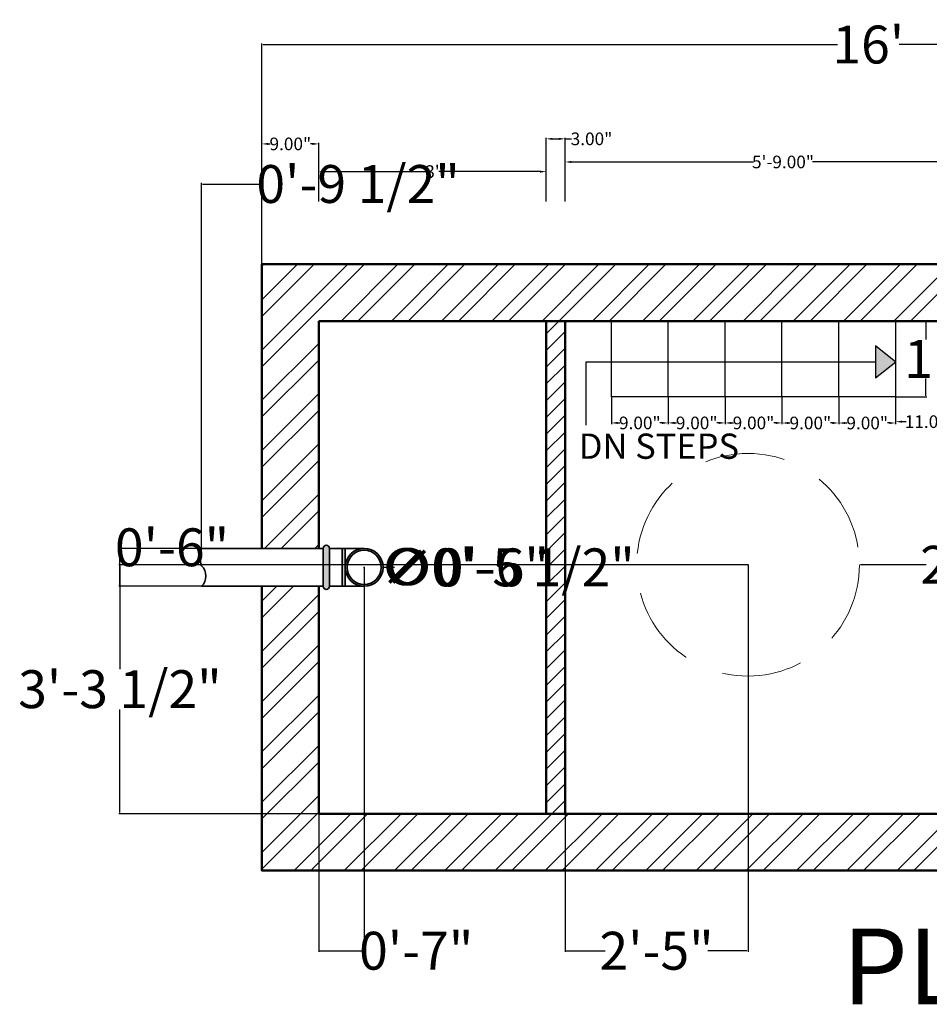
# Model space of a CAD drawing. Units: inches. Extents: x -34 to 285, y -151 to 155.
# Tile 5 of 10: x -15 to 129, y -1 to 155. Entities that reach past the tile are written whole.
import ezdxf

# ---------------------------------------------------------------- set-up
doc = ezdxf.new("R2010")
doc.units = ezdxf.units.IN
doc.header["$MEASUREMENT"] = 0
doc.linetypes.add('DASHED', pattern=[19.05, 12.7, -6.35])
for name, color, linetype, lineweight in [('A-ANNO-DIMS', 2, 'Continuous', 18), ('A-ANNO-TEXT', 7, 'Continuous', 25), ('A-DETL-HIDN', 8, 'DASHED', 18), ('A-FLOR-STRS', 3, 'Continuous', 25), ('A-WALL', 7, 'Continuous', 50), ('A-WALL-PATT', 8, 'Continuous', 18), ('P-SANR-PATT', 8, 'Continuous', 13), ('P-SANR-PIPE', 4, 'Continuous', 35)]:
    doc.layers.add(name, color=color, linetype=linetype, lineweight=lineweight)
doc.styles.get("Standard").update_dxf_attribs({"font": 'arial.ttf'})
doc.dimstyles.get("Standard").update_dxf_attribs({"dimtxt": 6, "dimasz": 0.18, "dimexe": 0.18, "dimexo": 0.0625, "dimgap": 0.09, "dimtad": 0, "dimtih": 1, "dimtoh": 1, "dimzin": 0, "dimdsep": 46, "dimlunit": 3, "dimtxsty": 'Standard', "dimcen": 0.09, "dimadec": 0, "dimazin": 0, "dimtfac": 1, "dimtofl": 0, "dimtmove": 0, "dimatfit": 3, "dimfxl": 1, "dimtolj": 1, "dimtzin": 0, "dimarcsym": 0})

# ---------------------------------------------------------------- blocks, each defined once
blk = doc.blocks.new('*D7')
at = {"layer": 'A-ANNO-DIMS', "color": 0, "lineweight": -2, "transparency": 16777216}
for p, q in [((123.25, 106.98), (128.12, 106.98)), ((127.94, 106.8), (127.94, 104.08)), ((127.94, 95.16), (127.94, 97.88)), ((123.25, 94.98), (128.12, 94.98))]:
    blk.add_line(p, q, dxfattribs=at)
at = {"layer": 'A-ANNO-DIMS', "color": 0, "transparency": 16777216}
for points in [[(127.91, 106.8), (127.97, 106.8), (127.94, 106.98)], [(127.91, 95.16), (127.97, 95.16), (127.94, 94.98)]]:
    blk.add_solid(points, dxfattribs=at)
at = {"layer": 'Defpoints', "color": 0, "transparency": 16777216}
for p in [(123.18, 106.98), (123.18, 94.98), (127.94, 94.98)]:
    blk.add_point(p, dxfattribs=at)
at = {"layer": 'A-ANNO-DIMS', "color": 0, "transparency": 16777216, "insert": (127.94, 100.98), "char_height": 6, "attachment_point": 5}
blk.add_mtext("\\A1;1'", dxfattribs=at)
blk = doc.blocks.new('*D8')
at = {"layer": 'A-ANNO-DIMS', "color": 0, "lineweight": -2, "transparency": 16777216}
for p, q in [((114.18, 94.92), (114.18, 90.66)), ((123.18, 94.92), (123.18, 90.66)), ((115.18, 90.84), (115.5, 90.84)), ((122.18, 90.84), (121.87, 90.84))]:
    blk.add_line(p, q, dxfattribs=at)
at = {"layer": 'A-ANNO-DIMS', "color": 0, "transparency": 16777216}
for points in [[(115.18, 91), (115.18, 90.67), (114.18, 90.84)], [(122.18, 91), (122.18, 90.67), (123.18, 90.84)]]:
    blk.add_solid(points, dxfattribs=at)
at = {"layer": 'Defpoints', "color": 0, "transparency": 16777216}
for p in [(114.18, 94.98), (123.18, 94.98), (114.18, 90.84)]:
    blk.add_point(p, dxfattribs=at)
at = {"layer": 'A-ANNO-DIMS', "color": 0, "transparency": 16777216, "insert": (118.68, 90.84), "char_height": 2, "attachment_point": 5}
blk.add_mtext('\\A1;9.00"', dxfattribs=at)
blk = doc.blocks.new('*D9')
at = {"layer": 'A-ANNO-DIMS', "color": 0, "lineweight": -2, "transparency": 16777216}
for p, q in [((105.18, 94.92), (105.18, 90.66)), ((114.18, 94.92), (114.18, 90.66)), ((106.18, 90.84), (106.5, 90.84)), ((113.18, 90.84), (112.87, 90.84))]:
    blk.add_line(p, q, dxfattribs=at)
at = {"layer": 'A-ANNO-DIMS', "color": 0, "transparency": 16777216}
for points in [[(106.18, 91), (106.18, 90.67), (105.18, 90.84)], [(113.18, 91), (113.18, 90.67), (114.18, 90.84)]]:
    blk.add_solid(points, dxfattribs=at)
at = {"layer": 'Defpoints', "color": 0, "transparency": 16777216}
for p in [(105.18, 94.98), (114.18, 94.98), (114.18, 90.84)]:
    blk.add_point(p, dxfattribs=at)
at = {"layer": 'A-ANNO-DIMS', "color": 0, "transparency": 16777216, "insert": (109.68, 90.84), "char_height": 2, "attachment_point": 5}
blk.add_mtext('\\A1;9.00"', dxfattribs=at)
blk = doc.blocks.new('*D10')
at = {"layer": 'A-ANNO-DIMS', "color": 0, "lineweight": -2, "transparency": 16777216}
for p, q in [((96.18, 94.92), (96.18, 90.67)), ((105.18, 94.92), (105.18, 90.67)), ((97.18, 90.85), (97.5, 90.85)), ((104.18, 90.85), (103.87, 90.85))]:
    blk.add_line(p, q, dxfattribs=at)
at = {"layer": 'A-ANNO-DIMS', "color": 0, "transparency": 16777216}
for points in [[(97.18, 91.02), (97.18, 90.68), (96.18, 90.85)], [(104.18, 91.02), (104.18, 90.68), (105.18, 90.85)]]:
    blk.add_solid(points, dxfattribs=at)
at = {"layer": 'Defpoints', "color": 0, "transparency": 16777216}
for p in [(96.18, 94.98), (105.18, 94.98), (96.18, 90.85)]:
    blk.add_point(p, dxfattribs=at)
at = {"layer": 'A-ANNO-DIMS', "color": 0, "transparency": 16777216, "insert": (100.68, 90.85), "char_height": 2, "attachment_point": 5}
blk.add_mtext('\\A1;9.00"', dxfattribs=at)
blk = doc.blocks.new('*D11')
at = {"layer": 'A-ANNO-DIMS', "color": 0, "lineweight": -2, "transparency": 16777216}
for p, q in [((87.18, 94.92), (87.18, 90.67)), ((96.18, 94.92), (96.18, 90.67)), ((88.18, 90.85), (88.5, 90.85)), ((95.18, 90.85), (94.87, 90.85))]:
    blk.add_line(p, q, dxfattribs=at)
at = {"layer": 'A-ANNO-DIMS', "color": 0, "transparency": 16777216}
for points in [[(88.18, 91.02), (88.18, 90.68), (87.18, 90.85)], [(95.18, 91.02), (95.18, 90.68), (96.18, 90.85)]]:
    blk.add_solid(points, dxfattribs=at)
at = {"layer": 'Defpoints', "color": 0, "transparency": 16777216}
for p in [(87.18, 94.98), (96.18, 94.98), (96.18, 90.85)]:
    blk.add_point(p, dxfattribs=at)
at = {"layer": 'A-ANNO-DIMS', "color": 0, "transparency": 16777216, "insert": (91.68, 90.85), "char_height": 2, "attachment_point": 5}
blk.add_mtext('\\A1;9.00"', dxfattribs=at)
blk = doc.blocks.new('*D12')
at = {"layer": 'A-ANNO-DIMS', "color": 0, "lineweight": -2, "transparency": 16777216}
for p, q in [((78.18, 94.92), (78.18, 90.67)), ((87.18, 94.92), (87.18, 90.67)), ((79.18, 90.85), (79.5, 90.85)), ((86.18, 90.85), (85.87, 90.85))]:
    blk.add_line(p, q, dxfattribs=at)
at = {"layer": 'A-ANNO-DIMS', "color": 0, "transparency": 16777216}
for points in [[(79.18, 91.02), (79.18, 90.68), (78.18, 90.85)], [(86.18, 91.02), (86.18, 90.68), (87.18, 90.85)]]:
    blk.add_solid(points, dxfattribs=at)
at = {"layer": 'Defpoints', "color": 0, "transparency": 16777216}
for p in [(78.18, 94.98), (87.18, 94.98), (78.18, 90.85)]:
    blk.add_point(p, dxfattribs=at)
at = {"layer": 'A-ANNO-DIMS', "color": 0, "transparency": 16777216, "insert": (82.68, 90.85), "char_height": 2, "attachment_point": 5}
blk.add_mtext('\\A1;9.00"', dxfattribs=at)
blk = doc.blocks.new('*D13')
at = {"layer": 'A-ANNO-DIMS', "color": 0, "lineweight": -2, "transparency": 16777216}
for p, q in [((123.18, 94.92), (123.18, 90.87)), ((134.18, 94.92), (134.18, 90.87)), ((124.18, 91.05), (124.82, 91.05)), ((133.18, 91.05), (132.55, 91.05))]:
    blk.add_line(p, q, dxfattribs=at)
at = {"layer": 'A-ANNO-DIMS', "color": 0, "transparency": 16777216}
for points in [[(124.18, 91.22), (124.18, 90.88), (123.18, 91.05)], [(133.18, 91.22), (133.18, 90.88), (134.18, 91.05)]]:
    blk.add_solid(points, dxfattribs=at)
at = {"layer": 'Defpoints', "color": 0, "transparency": 16777216}
for p in [(123.18, 94.98), (134.18, 94.98), (134.18, 91.05)]:
    blk.add_point(p, dxfattribs=at)
at = {"layer": 'A-ANNO-DIMS', "color": 0, "transparency": 16777216, "insert": (128.68, 91.05), "char_height": 2, "attachment_point": 5}
blk.add_mtext('\\A1;11.00"', dxfattribs=at)
blk = doc.blocks.new('*D14')
at = {"layer": 'A-ANNO-DIMS', "color": 0, "lineweight": -2, "transparency": 16777216}
for p, q in [((22.85, 125.9), (22.85, 135.21)), ((23.85, 135.03), (24.16, 135.03)), ((30.85, 135.03), (30.53, 135.03)), ((31.85, 125.9), (31.85, 135.21))]:
    blk.add_line(p, q, dxfattribs=at)
at = {"layer": 'A-ANNO-DIMS', "color": 0, "transparency": 16777216}
for points in [[(23.85, 135.2), (23.85, 134.86), (22.85, 135.03)], [(30.85, 135.2), (30.85, 134.86), (31.85, 135.03)]]:
    blk.add_solid(points, dxfattribs=at)
at = {"layer": 'Defpoints', "color": 0, "transparency": 16777216}
for p in [(31.85, 135.03), (22.85, 125.83), (31.85, 125.83)]:
    blk.add_point(p, dxfattribs=at)
at = {"layer": 'A-ANNO-DIMS', "color": 0, "transparency": 16777216, "insert": (27.35, 135.03), "char_height": 2, "attachment_point": 5}
blk.add_mtext('\\A1;9.00"', dxfattribs=at)
blk = doc.blocks.new('*D15')
at = {"layer": 'A-ANNO-DIMS', "color": 0, "lineweight": -2, "transparency": 16777216}
for p, q in [((31.85, 125.9), (31.85, 130.82)), ((32.85, 130.64), (48.84, 130.64)), ((66.85, 130.64), (50.86, 130.64)), ((67.85, 125.9), (67.85, 130.82))]:
    blk.add_line(p, q, dxfattribs=at)
at = {"layer": 'A-ANNO-DIMS', "color": 0, "transparency": 16777216}
for points in [[(32.85, 130.81), (32.85, 130.47), (31.85, 130.64)], [(66.85, 130.81), (66.85, 130.47), (67.85, 130.64)]]:
    blk.add_solid(points, dxfattribs=at)
at = {"layer": 'Defpoints', "color": 0, "transparency": 16777216}
for p in [(67.85, 130.64), (31.85, 125.83), (67.85, 125.83)]:
    blk.add_point(p, dxfattribs=at)
at = {"layer": 'A-ANNO-DIMS', "color": 0, "transparency": 16777216, "insert": (49.85, 130.64), "char_height": 2, "attachment_point": 5}
blk.add_mtext("\\A1;3'", dxfattribs=at)
blk = doc.blocks.new('*D16')
at = {"layer": 'A-ANNO-DIMS', "color": 0, "lineweight": -2, "transparency": 16777216}
for p, q in [((67.85, 125.9), (67.85, 136.01)), ((68.85, 135.83), (69.85, 135.83)), ((70.85, 125.9), (70.85, 136.01)), ((70.85, 135.83), (71.85, 135.83))]:
    blk.add_line(p, q, dxfattribs=at)
at = {"layer": 'A-ANNO-DIMS', "color": 0, "transparency": 16777216}
for points in [[(68.85, 135.99), (68.85, 135.66), (67.85, 135.83)], [(69.85, 135.99), (69.85, 135.66), (70.85, 135.83)]]:
    blk.add_solid(points, dxfattribs=at)
at = {"layer": 'Defpoints', "color": 0, "transparency": 16777216}
for p in [(70.85, 135.83), (67.85, 125.83), (70.85, 125.83)]:
    blk.add_point(p, dxfattribs=at)
at = {"layer": 'A-ANNO-DIMS', "color": 0, "transparency": 16777216, "insert": (75.03, 135.83), "char_height": 2, "attachment_point": 5}
blk.add_mtext('\\A1;3.00"', dxfattribs=at)
blk = doc.blocks.new('*D17')
at = {"layer": 'A-ANNO-DIMS', "color": 0, "lineweight": -2, "transparency": 16777216}
for p, q in [((70.85, 125.9), (70.85, 132.35)), ((71.85, 132.17), (100.66, 132.17)), ((138.85, 132.17), (110.04, 132.17)), ((139.85, 125.9), (139.85, 132.35))]:
    blk.add_line(p, q, dxfattribs=at)
at = {"layer": 'A-ANNO-DIMS', "color": 0, "transparency": 16777216}
for points in [[(71.85, 132.33), (71.85, 132), (70.85, 132.17)], [(138.85, 132.33), (138.85, 132), (139.85, 132.17)]]:
    blk.add_solid(points, dxfattribs=at)
at = {"layer": 'Defpoints', "color": 0, "transparency": 16777216}
for p in [(139.85, 132.17), (70.85, 125.83), (139.85, 125.83)]:
    blk.add_point(p, dxfattribs=at)
at = {"layer": 'A-ANNO-DIMS', "color": 0, "transparency": 16777216, "insert": (105.35, 132.17), "char_height": 2, "attachment_point": 5}
blk.add_mtext('\\A1;5\'-9.00"', dxfattribs=at)
blk = doc.blocks.new('*D21')
at = {"layer": 'A-ANNO-DIMS', "color": 0, "lineweight": -2, "transparency": 16777216}
for p, q in [((22.85, 130.62), (22.85, 150.94)), ((23.03, 150.76), (113.95, 150.76)), ((214.67, 150.76), (123.74, 150.76)), ((214.85, 127.74), (214.85, 150.94))]:
    blk.add_line(p, q, dxfattribs=at)
at = {"layer": 'A-ANNO-DIMS', "color": 0, "transparency": 16777216}
for points in [[(23.03, 150.79), (23.03, 150.73), (22.85, 150.76)], [(214.67, 150.79), (214.67, 150.73), (214.85, 150.76)]]:
    blk.add_solid(points, dxfattribs=at)
at = {"layer": 'Defpoints', "color": 0, "transparency": 16777216}
for p in [(22.85, 150.76), (22.85, 130.55), (214.85, 127.68)]:
    blk.add_point(p, dxfattribs=at)
at = {"layer": 'A-ANNO-DIMS', "color": 0, "transparency": 16777216, "insert": (118.85, 150.76), "char_height": 6, "attachment_point": 5}
blk.add_mtext("\\A1;16'", dxfattribs=at)
blk = doc.blocks.new('*D40')
at = {"layer": 'A-ANNO-DIMS', "color": 0, "lineweight": -2, "transparency": 16777216}
for p, q in [((99.81, 68.33), (99.81, 7.1)), ((70.85, 28.92), (70.85, 7.1)), ((71.03, 7.28), (77.21, 7.28)), ((99.63, 7.28), (93.45, 7.28))]:
    blk.add_line(p, q, dxfattribs=at)
at = {"layer": 'A-ANNO-DIMS', "color": 0, "transparency": 16777216}
for points in [[(71.03, 7.31), (71.03, 7.25), (70.85, 7.28)], [(99.63, 7.31), (99.63, 7.25), (99.81, 7.28)]]:
    blk.add_solid(points, dxfattribs=at)
at = {"layer": 'Defpoints', "color": 0, "transparency": 16777216}
for p in [(99.81, 68.39), (70.85, 28.98), (99.81, 7.28)]:
    blk.add_point(p, dxfattribs=at)
at = {"layer": 'A-ANNO-DIMS', "color": 0, "transparency": 16777216, "insert": (85.33, 7.28), "char_height": 6, "attachment_point": 5}
blk.add_mtext('\\A1;2\'-5"', dxfattribs=at)
blk = doc.blocks.new('*D42')
at = {"layer": 'A-ANNO-DIMS', "color": 0, "lineweight": -2, "transparency": 16777216}
for p, q in [((99.75, 68.39), (0.19, 68.39)), ((0.37, 68.21), (0.37, 51.88)), ((0.37, 29.16), (0.37, 45.49)), ((70.78, 28.98), (0.19, 28.98))]:
    blk.add_line(p, q, dxfattribs=at)
at = {"layer": 'A-ANNO-DIMS', "color": 0, "transparency": 16777216}
for points in [[(0.34, 68.21), (0.4, 68.21), (0.37, 68.39)], [(0.34, 29.16), (0.4, 29.16), (0.37, 28.98)]]:
    blk.add_solid(points, dxfattribs=at)
at = {"layer": 'Defpoints', "color": 0, "transparency": 16777216}
for p in [(0.37, 68.39), (99.81, 68.39), (70.85, 28.98)]:
    blk.add_point(p, dxfattribs=at)
at = {"layer": 'A-ANNO-DIMS', "color": 0, "transparency": 16777216, "insert": (0.37, 48.69), "char_height": 6, "attachment_point": 5}
blk.add_mtext('\\A1;3\'-3 1/2"', dxfattribs=at)
blk = doc.blocks.new('*D43')
at = {"layer": 'A-ANNO-DIMS', "color": 0, "lineweight": -2, "transparency": 16777216}
for p, q in [((39.04, 67.92), (39.04, 7.1)), ((31.85, 28.92), (31.85, 7.1)), ((32.03, 7.28), (38.86, 7.28)), ((39.04, 7.28), (39.22, 7.28))]:
    blk.add_line(p, q, dxfattribs=at)
at = {"layer": 'A-ANNO-DIMS', "color": 0, "transparency": 16777216}
for points in [[(32.03, 7.31), (32.03, 7.25), (31.85, 7.28)], [(38.86, 7.31), (38.86, 7.25), (39.04, 7.28)]]:
    blk.add_solid(points, dxfattribs=at)
at = {"layer": 'Defpoints', "color": 0, "transparency": 16777216}
for p in [(39.04, 67.98), (31.85, 28.98), (39.04, 7.28)]:
    blk.add_point(p, dxfattribs=at)
at = {"layer": 'A-ANNO-DIMS', "color": 0, "transparency": 16777216, "insert": (47.28, 7.28), "char_height": 6, "attachment_point": 5}
blk.add_mtext('\\A1;0\'-7"', dxfattribs=at)
blk = doc.blocks.new('*D46')
at = {"layer": 'A-ANNO-DIMS', "color": 0, "lineweight": -2, "transparency": 16777216}
for p, q in [((13.22, 70.98), (0.19, 70.98)), ((0.37, 70.98), (0.37, 71.16)), ((0.37, 71.16), (0.55, 71.16)), ((0.37, 65.16), (0.37, 70.8)), ((13.22, 64.98), (0.19, 64.98))]:
    blk.add_line(p, q, dxfattribs=at)
at = {"layer": 'A-ANNO-DIMS', "color": 0, "transparency": 16777216}
for points in [[(0.34, 70.8), (0.4, 70.8), (0.37, 70.98)], [(0.34, 65.16), (0.4, 65.16), (0.37, 64.98)]]:
    blk.add_solid(points, dxfattribs=at)
at = {"layer": 'Defpoints', "color": 0, "transparency": 16777216}
for p in [(0.37, 70.98), (13.29, 70.98), (13.29, 64.98)]:
    blk.add_point(p, dxfattribs=at)
at = {"layer": 'A-ANNO-DIMS', "color": 0, "transparency": 16777216, "insert": (8.62, 71.16), "char_height": 6, "attachment_point": 5}
blk.add_mtext('\\A1;0\'-6"', dxfattribs=at)
blk = doc.blocks.new('*D47')
at = {"layer": 'A-ANNO-DIMS', "color": 0, "lineweight": -2, "transparency": 16777216}
for p, q in [((13.29, 71.04), (13.29, 128.86)), ((13.47, 128.68), (22.67, 128.68)), ((22.85, 71.04), (22.85, 128.86)), ((22.85, 128.68), (23.03, 128.68))]:
    blk.add_line(p, q, dxfattribs=at)
at = {"layer": 'A-ANNO-DIMS', "color": 0, "transparency": 16777216}
for points in [[(13.47, 128.71), (13.47, 128.65), (13.29, 128.68)], [(22.67, 128.71), (22.67, 128.65), (22.85, 128.68)]]:
    blk.add_solid(points, dxfattribs=at)
at = {"layer": 'Defpoints', "color": 0, "transparency": 16777216}
for p in [(22.85, 128.68), (13.29, 70.98), (22.85, 70.98)]:
    blk.add_point(p, dxfattribs=at)
at = {"layer": 'A-ANNO-DIMS', "color": 0, "transparency": 16777216, "insert": (38.08, 128.68), "char_height": 6, "attachment_point": 5}
blk.add_mtext('\\A1;0\'-9 1/2"', dxfattribs=at)
blk = doc.blocks.new('*D88')
at = {"layer": 'A-ANNO-DIMS', "color": 0, "lineweight": -2, "transparency": 16777216}
for p, q in [((99.72, 68.39), (99.9, 68.39)), ((99.81, 68.3), (99.81, 68.48)), ((128.01, 68.39), (117.62, 68.39))]:
    blk.add_line(p, q, dxfattribs=at)
at = {"layer": 'A-ANNO-DIMS', "color": 0, "transparency": 16777216}
blk.add_solid([(117.62, 68.42), (117.62, 68.36), (117.44, 68.39)], dxfattribs=at)
at = {"layer": 'Defpoints', "color": 0, "transparency": 16777216}
for p in [(82.19, 68.39), (117.44, 68.39)]:
    blk.add_point(p, dxfattribs=at)
at = {"layer": 'A-ANNO-DIMS', "color": 0, "transparency": 16777216, "insert": (148.01, 68.39), "char_height": 6, "attachment_point": 5}
blk.add_mtext('\\A1;2X ∅2\'-11"', dxfattribs=at)
blk = doc.blocks.new('*D89')
at = {"layer": 'A-ANNO-DIMS', "color": 0, "lineweight": -2, "transparency": 16777216}
for p, q in [((38.95, 67.98), (39.13, 67.98)), ((39.04, 67.89), (39.04, 68.07)), ((43.84, 67.98), (42.22, 67.98))]:
    blk.add_line(p, q, dxfattribs=at)
at = {"layer": 'A-ANNO-DIMS', "color": 0, "transparency": 16777216}
blk.add_solid([(42.22, 68.01), (42.22, 67.95), (42.04, 67.98)], dxfattribs=at)
at = {"layer": 'Defpoints', "color": 0, "transparency": 16777216}
for p in [(36.04, 67.98), (42.04, 67.98)]:
    blk.add_point(p, dxfattribs=at)
at = {"layer": 'A-ANNO-DIMS', "color": 0, "transparency": 16777216, "insert": (55.16, 67.98), "char_height": 6, "attachment_point": 5}
blk.add_mtext('\\A1;∅0\'-6"', dxfattribs=at)
blk = doc.blocks.new('*D90')
at = {"layer": 'A-ANNO-DIMS', "color": 0, "lineweight": -2, "transparency": 16777216}
for p, q in [((38.95, 67.98), (39.13, 67.98)), ((39.04, 67.89), (39.04, 68.07)), ((43.36, 67.98), (41.92, 67.98))]:
    blk.add_line(p, q, dxfattribs=at)
at = {"layer": 'A-ANNO-DIMS', "color": 0, "transparency": 16777216}
blk.add_solid([(41.92, 68.01), (41.92, 67.95), (41.74, 67.98)], dxfattribs=at)
at = {"layer": 'Defpoints', "color": 0, "transparency": 16777216}
for p in [(36.34, 67.98), (41.74, 67.98)]:
    blk.add_point(p, dxfattribs=at)
at = {"layer": 'A-ANNO-DIMS', "color": 0, "transparency": 16777216, "insert": (61.68, 67.98), "char_height": 6, "attachment_point": 5}
blk.add_mtext('\\A1;∅0\'-5 1/2"', dxfattribs=at)

msp = doc.modelspace()

# ---------------------------------------------------------------- hatches: boundary and pattern name
at = {"layer": 'A-FLOR-STRS'}
h = msp.add_hatch(color=256, dxfattribs=at)
h.dxf.hatch_style = 1
h.paths.add_polyline_path([(123.184, 100.48), (120.012, 103.037), (120.012, 97.923)])
at = {"layer": 'A-WALL-PATT'}
h = msp.add_hatch(dxfattribs=at)
h.set_pattern_fill('ANSI32', color=256, scale=15)
h.paths.add_polyline_path([(214.846, 64.981), (205.846, 64.981), (205.846, 64.112), (205.846, 28.981), (31.846, 28.981), (31.846, 64.981), (22.846, 64.981), (22.846, 19.981), (214.846, 19.981)])
h.paths.add_polyline_path([(67.846, 106.981), (67.846, 115.981), (22.846, 115.981), (22.846, 70.981), (31.846, 70.981), (31.846, 106.981)])
h = msp.add_hatch(dxfattribs=at)
h.set_pattern_fill('ANSI32', color=256, scale=15)
h.paths.add_polyline_path([(214.846, 115.981), (22.846, 115.981), (22.846, 70.981), (31.846, 70.981), (31.846, 106.981), (205.846, 106.981), (205.846, 70.981), (214.846, 70.981)])
h = msp.add_hatch(dxfattribs=at)
h.set_pattern_fill('ANSI31', color=256, scale=15)
h.paths.add_polyline_path([(70.846, 106.981), (67.846, 106.981), (67.846, 28.981), (70.846, 28.981)])
at = {"layer": 'P-SANR-PATT'}
h = msp.add_hatch(color=256, dxfattribs=at)
h.dxf.hatch_style = 1
h.paths.add_polyline_path([(33.536, 70.981, 1), (32.536, 70.981), (32.536, 64.981, 1), (33.536, 64.981)])
h = msp.add_hatch(color=256, dxfattribs=at)
h.dxf.hatch_style = 1
h.paths.add_polyline_path([(36.036, 70.981), (35.536, 70.981), (35.536, 64.981), (36.036, 64.981)])
h = msp.add_hatch(color=256, dxfattribs=at)
h.dxf.hatch_style = 1
h.paths.add_polyline_path([(36.036, 67.981, 1), (42.036, 67.981, 1)])
h.paths.add_polyline_path([(41.736, 67.981, -1), (36.336, 67.981, -1)], flags=16)

# ---------------------------------------------------------------- linework, layer by layer
at = {"layer": 'A-DETL-HIDN'}
msp.add_circle((99.814, 68.391), 17.624, dxfattribs=at)
at = {"layer": 'A-FLOR-STRS'}
for p, q in [((78.184, 94.981), (78.184, 106.981)), ((87.184, 94.981), (87.184, 106.981)), ((96.184, 94.981), (96.184, 106.981)), ((105.184, 94.981), (105.184, 106.981)), ((114.184, 94.981), (114.184, 106.981)), ((123.184, 94.981), (123.184, 106.981)), ((123.184, 100.48), (120.012, 103.037)), ((120.012, 103.037), (120.012, 97.923)), ((120.012, 100.48), (74.124, 100.48)), ((74.124, 100.48), (74.124, 90.5)), ((123.184, 100.48), (120.012, 97.923))]:
    msp.add_line(p, q, dxfattribs=at)
msp.add_lwpolyline([(123.184, 94.981), (78.184, 94.981)], dxfattribs=at)
at = {"layer": 'A-WALL'}
for points in [[(22.846, 64.981), (22.846, 19.981), (214.846, 19.981), (214.846, 115.981), (22.846, 115.981), (22.846, 70.981)], [(31.846, 106.981), (31.846, 70.981)], [(205.846, 106.981), (31.846, 106.981)], [(67.846, 106.981), (67.846, 28.981)], [(70.846, 106.981), (70.846, 28.981)], [(31.846, 64.981), (31.846, 28.981)], [(31.846, 28.981), (214.846, 28.981)]]:
    msp.add_lwpolyline(points, dxfattribs=at)
at = {"layer": 'P-SANR-PIPE'}
for p, q in [((22.846, 70.981), (32.536, 70.981)), ((32.536, 70.981), (32.536, 64.981)), ((33.536, 70.981), (33.536, 64.981)), ((33.536, 70.981), (39.036, 70.981)), ((35.536, 70.981), (35.536, 64.981)), ((36.036, 70.981), (36.036, 64.981)), ((22.846, 64.981), (32.536, 64.981)), ((33.536, 64.981), (39.036, 64.981))]:
    msp.add_line(p, q, dxfattribs=at)
msp.add_lwpolyline([(13.286, 64.981, 0.4260379), (13.3, 68.24, -0.1623), (13.286, 70.981)], format="xyb", dxfattribs=at)
for points in [[(22.846, 70.981), (13.286, 70.981)], [(13.286, 64.981), (22.846, 64.981)]]:
    msp.add_lwpolyline(points, dxfattribs=at)
for radius in [3, 2.7]:
    msp.add_circle((39.036, 67.981), radius, dxfattribs=at)
for centre, start, end in [((33.036, 70.981), 0, 180), ((33.036, 64.981), 180, 0)]:
    msp.add_arc(centre, 0.5, start, end, dxfattribs=at)

# ---------------------------------------------------------------- texts
at = {"layer": 'A-ANNO-TEXT', "attachment_point": 1}
for s, insert, char_height in [('DN STEPS', (73.024, 89.167), 4), ('PLAN ', (114.748, 10.798), 12)]:
    msp.add_mtext_dynamic_manual_height_columns(s, width=53.60251, gutter_width=1, heights=[0], dxfattribs=dict(at, insert=insert, char_height=char_height))

# ---------------------------------------------------------------- dimensions: what is measured, and where the dimension line sits
at = {"layer": 'A-ANNO-DIMS'}
for base, p1, p2, override, picture, middle in [((22.846, 150.759), (214.846, 127.681), (22.846, 130.553), {"dimclrd": 0, "dimclre": 0, "dimclrt": 0}, '*D21', (118.846, 150.759)), ((22.846, 128.681), (13.286, 70.981), (22.846, 70.981), {"dimdec": 1, "dimlfac": 1, "dimrnd": 0, "dimzin": 1, "dimdsep": 46, "dimlunit": 4, "dimfrac": 2}, '*D47', (38.081, 128.681)), ((31.846, 135.03), (22.846, 125.833), (31.846, 125.833), {"dimtxt": 2, "dimasz": 1, "dimclrd": 0, "dimclre": 0, "dimclrt": 0}, '*D14', (27.346, 135.03)), ((70.846, 135.828), (67.846, 125.833), (70.846, 125.833), {"dimtxt": 2, "dimasz": 1, "dimclrd": 0, "dimclre": 0, "dimclrt": 0}, '*D16', (75.026, 135.828)), ((139.846, 132.167), (70.846, 125.833), (139.846, 125.833), {"dimtxt": 2, "dimasz": 1, "dimclrd": 0, "dimclre": 0, "dimclrt": 0}, '*D17', (105.346, 132.167)), ((67.846, 130.641), (31.846, 125.833), (67.846, 125.833), {"dimtxt": 2, "dimasz": 1, "dimclrd": 0, "dimclre": 0, "dimclrt": 0}, '*D15', (49.846, 130.641)), ((78.184, 90.851), (87.184, 94.981), (78.184, 94.981), {"dimtxt": 2, "dimasz": 1, "dimclrd": 0, "dimclre": 0, "dimclrt": 0}, '*D12', (82.684, 90.851)), ((96.184, 90.851), (87.184, 94.981), (96.184, 94.981), {"dimtxt": 2, "dimasz": 1, "dimclrd": 0, "dimclre": 0, "dimclrt": 0}, '*D11', (91.684, 90.851)), ((96.184, 90.851), (105.184, 94.981), (96.184, 94.981), {"dimtxt": 2, "dimasz": 1, "dimclrd": 0, "dimclre": 0, "dimclrt": 0}, '*D10', (100.684, 90.851)), ((114.184, 90.836), (105.184, 94.981), (114.184, 94.981), {"dimtxt": 2, "dimasz": 1, "dimclrd": 0, "dimclre": 0, "dimclrt": 0}, '*D9', (109.684, 90.836)), ((114.184, 90.836), (123.184, 94.981), (114.184, 94.981), {"dimtxt": 2, "dimasz": 1, "dimclrd": 0, "dimclre": 0, "dimclrt": 0}, '*D8', (118.684, 90.836)), ((134.184, 91.051), (123.184, 94.981), (134.184, 94.981), {"dimtxt": 2, "dimasz": 1, "dimclrd": 0, "dimclre": 0, "dimclrt": 0}, '*D13', (128.684, 91.051)), ((39.036, 7.281), (31.846, 28.981), (39.036, 67.981), {"dimdec": 1, "dimlfac": 1, "dimrnd": 0, "dimzin": 1, "dimdsep": 46, "dimlunit": 4, "dimfrac": 2}, '*D43', (47.281, 7.281)), ((99.814, 7.281), (70.846, 28.981), (99.814, 68.391), {"dimdec": 1, "dimlfac": 1, "dimrnd": 0, "dimzin": 1, "dimdsep": 46, "dimlunit": 4, "dimfrac": 2}, '*D40', (85.33, 7.281))]:
    dim = msp.add_linear_dim(base=base, p1=p1, p2=p2, dimstyle='Standard', override=override, dxfattribs=at)
    dim.commit()
    dim.dimension.update_dxf_attribs({"geometry": picture, "text_midpoint": middle})
for base, p1, p2, override, picture, middle in [((127.945, 94.981), (123.184, 106.981), (123.184, 94.981), {"dimclrd": 0, "dimclre": 0, "dimclrt": 0}, '*D7', (127.945, 100.981)), ((0.371, 70.981), (13.286, 64.981), (13.286, 70.981), {"dimdec": 1, "dimlfac": 1, "dimrnd": 0, "dimzin": 1, "dimdsep": 46, "dimlunit": 4, "dimfrac": 2}, '*D46', (8.615, 71.161)), ((0.371, 68.391), (70.846, 28.981), (99.814, 68.391), {"dimdec": 1, "dimlfac": 1, "dimrnd": 0, "dimzin": 1, "dimdsep": 46, "dimlunit": 4, "dimfrac": 2}, '*D42', (0.371, 48.686))]:
    dim = msp.add_linear_dim(base=base, p1=p1, p2=p2, angle=90, dimstyle='Standard', override=override, dxfattribs=at)
    dim.commit()
    dim.dimension.update_dxf_attribs({"geometry": picture, "text_midpoint": middle})
for p1, p2, picture, middle in [((36.336, 67.98), (41.736, 67.981), '*D90', (43.356, 67.981)), ((36.036, 67.98), (42.036, 67.981), '*D89', (43.836, 67.981))]:
    dim = msp.add_diameter_dim_2p(p1=p1, p2=p2, dimstyle='Standard', override={"dimdec": 1, "dimlfac": 1, "dimrnd": 0, "dimzin": 1, "dimdsep": 46, "dimlunit": 4, "dimfrac": 2}, dxfattribs=at)
    dim.commit()
    dim.dimension.update_dxf_attribs({"geometry": picture, "text_midpoint": middle, "dimtype": 163})
dim = msp.add_diameter_dim_2p(p1=(82.19, 68.39), p2=(117.439, 68.391), text='2X <>', dimstyle='Standard', override={"dimdec": 1, "dimlfac": 1, "dimrnd": 0, "dimzin": 1, "dimdsep": 46, "dimlunit": 4, "dimfrac": 2}, dxfattribs=at)
dim.commit()
dim.dimension.update_dxf_attribs({"geometry": '*D88', "text_midpoint": (128.013, 68.391), "dimtype": 163})

doc.saveas('drawing.dxf')
